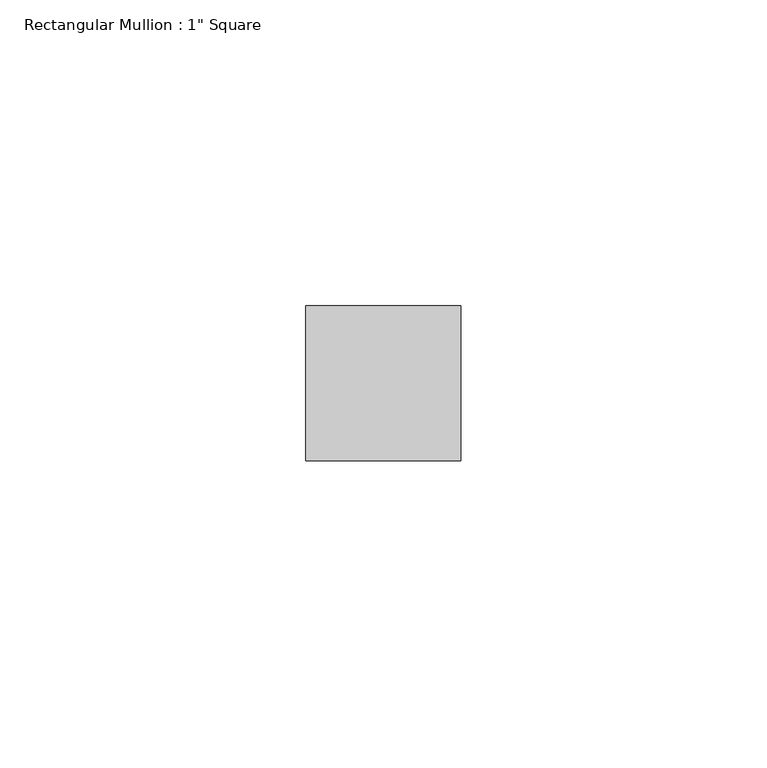
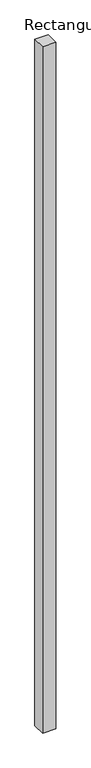
"""IFC4 building model written with IfcOpenShell, lengths in millimetres: member geometry."""

from ifc_helpers import new_model, si_unit, frame, origin, place, context, project, spatial, polyline, outline, extrude, source, transform, mapped, element, save


def member_20a2445f(model_context):
    return source(origin(), model_context, "Body", "SweptSolid", [
        extrude(outline(polyline([(0.0, 12.7), (0.0, -12.7), (-25.4, -12.7), (-25.4, 12.7), (0.0, 12.7)])), frame((0.0, 0.0, -1397.0), z_axis=(0.0, 0.0, 1.0), x_axis=(1.0, 0.0, 0.0)), (0.0, 0.0, 1.0), 1397.0),
    ])


if __name__ == "__main__":
    model = new_model("IFC4")
    model_context = context("Model", 3, world=origin())
    ifc_project = project(units=[si_unit("LENGTHUNIT", "METRE", prefix="MILLI")], contexts=[model_context])
    site = spatial("IfcSite", under=ifc_project)
    building = spatial("IfcBuilding", under=site)
    placement = place(None, origin())
    member_shape = member_20a2445f(model_context)
    element("IfcMember", 1, ObjectType="Rectangular Mullion : 1\" Square", at=placement, inside=building, context=model_context, shape_type="MappedRepresentation", body=[
        mapped(member_shape, transform((0.0, 0.0, 0.0), x_axis=(1.0, 0.0, 0.0), y_axis=(0.0, 1.0, 0.0), z_axis=(0.0, 0.0, 1.0))),
    ])
    save(model, "model.ifc")

# Revit data of these elements
# Type "Rectangular Mullion : 1\" Square"
#   built-in parameter 1007304 = 0.0833333 (stored number, unit not read)
#   built-in parameter 1007301 = 0.0416667 (stored number, unit not read)
#   built-in parameter 1007300 = 0.0416667 (stored number, unit not read)
